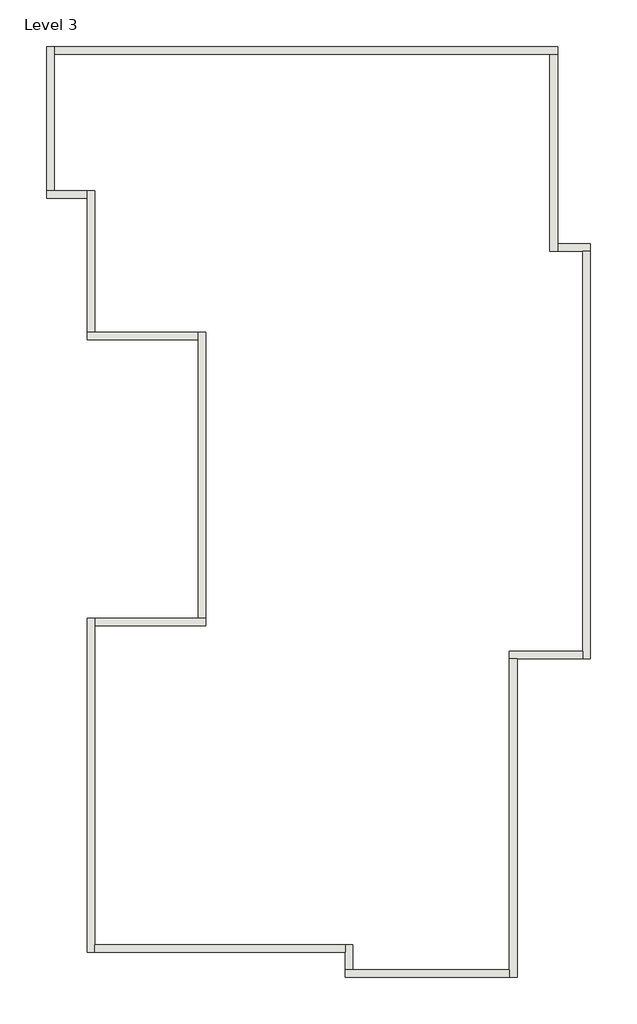
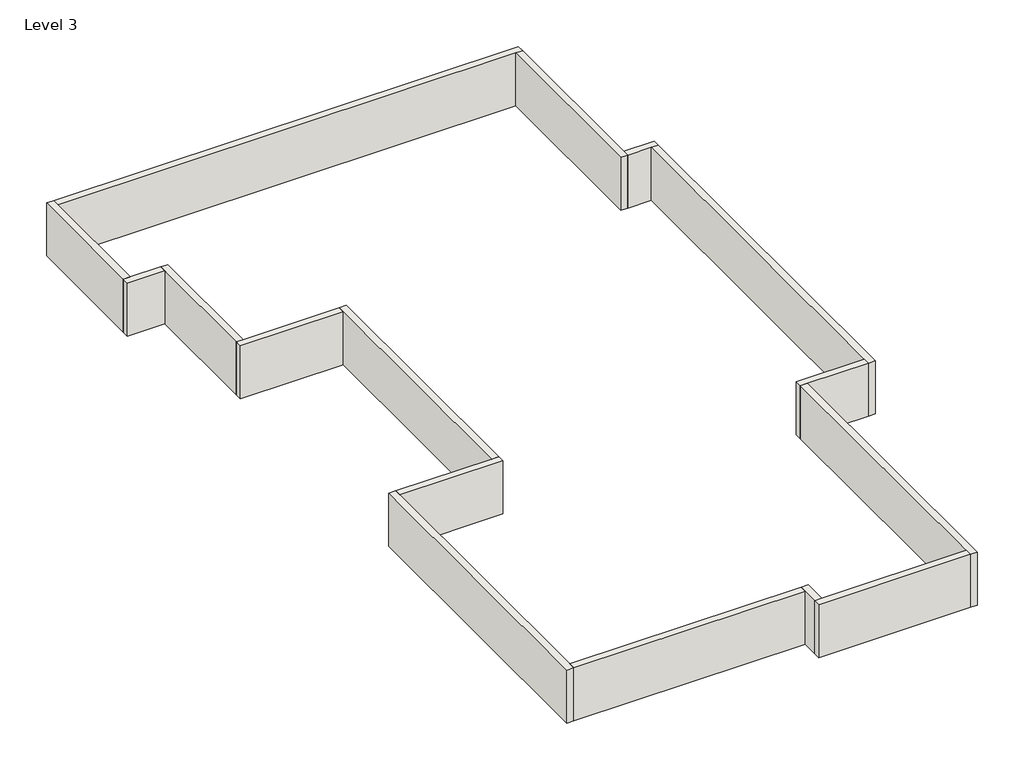
# One storey: 16 walls.
"""IFC4 building model written with IfcOpenShell, lengths in millimetres."""

from ifc_helpers import new_model, si_unit, frame, origin, place, context, project, spatial, polyline, outline, extrude, faceted_brep, element, save

model = new_model("IFC4")

# Units and contexts
model_context = context("Model", 3, world=origin())
ifc_project = project(units=[si_unit("LENGTHUNIT", "METRE", prefix="MILLI")], contexts=[model_context])

# Site, building, storey
site = spatial("IfcSite", under=ifc_project)
building = spatial("IfcBuilding", under=site)
storey = spatial("IfcBuildingStorey", under=building, Name="Level 3", Elevation=6400.8)

# Walls
placement = place(None, origin())
element("IfcWall", 1, ObjectType="Generic - 4.5\"", at=placement, inside=storey, context=model_context, shape_type="Brep", body=[
    faceted_brep([(-6988.9378503, -5768.8887643, 6400.8), (-6988.9378503, -5654.5887643, 6400.8), (-6988.9378503, -853.9864583, 6400.8), (-6988.9378503, -739.6864583, 6400.8), (-6988.9378503, -739.6864583, 7315.2), (-6988.9378503, -853.9864583, 7315.2), (-6988.9378503, -5654.5887643, 7315.2), (-6988.9378503, -5768.8887643, 7315.2), (-7103.2378503, -5768.8864583, 6400.8), (-7103.2378503, -5768.8864583, 7315.2), (-7103.2378503, -739.6864583, 7315.2), (-7103.2378503, -739.6864583, 6400.8)], [[[0, 1, 2, 3, 4, 5, 6, 7]], [[8, 9, 10, 11]], [[3, 2, 1, 0, 8, 11]], [[7, 6, 5, 4, 10, 9]], [[4, 3, 11, 10]], [[0, 7, 9, 8]]]),
])
element("IfcWall", 2, ObjectType="Generic - 4.5\"", at=placement, inside=storey, context=model_context, shape_type="Brep", body=[
    faceted_brep([(-6988.9378503, -853.9864583, 6400.8), (-5312.0457903, -853.9864583, 6400.8), (-5312.0457903, -853.9864583, 7315.2), (-6988.9378503, -853.9864583, 7315.2), (-6988.9378503, -739.6864583, 6400.8), (-6988.9378503, -739.6864583, 7315.2), (-5426.3457903, -739.6864583, 7315.2), (-5312.0457903, -739.6864583, 7315.2), (-5312.0457903, -739.6864583, 6400.8), (-5426.3457903, -739.6864583, 6400.8)], [[[0, 1, 2, 3]], [[4, 5, 6, 7, 8, 9]], [[1, 0, 4, 9, 8]], [[3, 2, 7, 6, 5]], [[0, 3, 5, 4]], [[2, 1, 8, 7]]]),
])
element("IfcWall", 3, ObjectType="Generic - 4.5\"", at=placement, inside=storey, context=model_context, shape_type="Brep", body=[
    faceted_brep([(-5312.0457903, -739.6864583, 6400.8), (-5312.0457903, 3565.6135417, 6400.8), (-5312.0457903, 3565.6135417, 7315.2), (-5312.0457903, -739.6864583, 7315.2), (-5426.3457903, -739.6864583, 6400.8), (-5426.3457903, -739.6864583, 7315.2), (-5426.3457903, 3451.3135417, 7315.2), (-5426.3457903, 3565.6135417, 7315.2), (-5426.3457903, 3565.6135417, 6400.8), (-5426.3457903, 3451.3135417, 6400.8)], [[[0, 1, 2, 3]], [[4, 5, 6, 7, 8, 9]], [[1, 0, 4, 9, 8]], [[3, 2, 7, 6, 5]], [[0, 3, 5, 4]], [[2, 1, 8, 7]]]),
])
element("IfcWall", 4, ObjectType="Generic - 4.5\"", at=placement, inside=storey, context=model_context, shape_type="Brep", body=[
    faceted_brep([(-5426.3457903, 3565.6135417, 6400.8), (-6988.9378503, 3565.6135417, 6400.8), (-7103.2378503, 3565.6135417, 6400.8), (-7103.2378503, 3565.6135417, 7315.2), (-6988.9378503, 3565.6135417, 7315.2), (-5426.3457903, 3565.6135417, 7315.2), (-5426.3457903, 3451.3135417, 6400.8), (-5426.3457903, 3451.3135417, 7315.2), (-7103.2378503, 3451.3135417, 7315.2), (-7103.2378503, 3451.3135417, 6400.8)], [[[0, 1, 2, 3, 4, 5]], [[6, 7, 8, 9]], [[2, 1, 0, 6, 9]], [[5, 4, 3, 8, 7]], [[0, 5, 7, 6]], [[3, 2, 9, 8]]]),
])
element("IfcWall", 5, ObjectType="Generic - 4.5\"", at=placement, inside=storey, context=model_context, shape_type="Brep", body=[
    faceted_brep([(-6988.9378503, 3565.6135417, 6400.8), (-6988.9378503, 5699.2135417, 6400.8), (-6988.9378503, 5699.2135417, 7315.2), (-6988.9378503, 3565.6135417, 7315.2), (-7103.2378503, 3565.6135417, 6400.8), (-7103.2378503, 3565.6135417, 7315.2), (-7103.2378503, 5584.9135417, 7315.2), (-7103.2378503, 5699.2135417, 7315.2), (-7103.2378503, 5699.2135417, 6400.8), (-7103.2378503, 5584.9135417, 6400.8)], [[[0, 1, 2, 3]], [[4, 5, 6, 7, 8, 9]], [[1, 0, 4, 9, 8]], [[3, 2, 7, 6, 5]], [[0, 3, 5, 4]], [[2, 1, 8, 7]]]),
])
element("IfcWall", 6, ObjectType="Generic - 4.5\"", at=placement, inside=storey, context=model_context, shape_type="Brep", body=[
    faceted_brep([(-7103.2378503, 5699.2135417, 6400.8), (-7598.5378503, 5699.2135417, 6400.8), (-7712.8378503, 5699.2135417, 6400.8), (-7712.8378503, 5699.2135417, 7315.2), (-7598.5378503, 5699.2135417, 7315.2), (-7103.2378503, 5699.2135417, 7315.2), (-7103.2378503, 5584.9135417, 6400.8), (-7103.2378503, 5584.9135417, 7315.2), (-7712.8378503, 5584.9135417, 7315.2), (-7712.8378503, 5584.9135417, 6400.8)], [[[0, 1, 2, 3, 4, 5]], [[6, 7, 8, 9]], [[2, 1, 0, 6, 9]], [[5, 4, 3, 8, 7]], [[0, 5, 7, 6]], [[3, 2, 9, 8]]]),
])
element("IfcWall", 7, ObjectType="Generic - 4.5\"", at=placement, inside=storey, context=model_context, shape_type="Brep", body=[
    faceted_brep([(-7598.5378503, 5699.2135417, 6400.8), (-7598.5378503, 7756.6135417, 6400.8), (-7598.5378503, 7870.9135417, 6400.8), (-7598.5378503, 7870.9135417, 7315.2), (-7598.5378503, 7756.6135417, 7315.2), (-7598.5378503, 5699.2135417, 7315.2), (-7712.8378503, 5699.2135417, 6400.8), (-7712.8378503, 5699.2135417, 7315.2), (-7712.8378503, 7870.9135417, 7315.2), (-7712.8378503, 7870.9135417, 6400.8)], [[[0, 1, 2, 3, 4, 5]], [[6, 7, 8, 9]], [[2, 1, 0, 6, 9]], [[5, 4, 3, 8, 7]], [[0, 5, 7, 6]], [[3, 2, 9, 8]]]),
])
element("IfcWall", 8, ObjectType="Generic - 4.5\"", at=placement, inside=storey, context=model_context, shape_type="Brep", body=[
    faceted_brep([(-7598.5378503, 7756.6135417, 6400.8), (-130.9378503, 7756.6135417, 6400.8), (-16.6378503, 7756.6135417, 6400.8), (-16.6378503, 7756.6135417, 7315.2), (-130.9378503, 7756.6135417, 7315.2), (-7598.5378503, 7756.6135417, 7315.2), (-7598.5378503, 7870.9135417, 6400.8), (-7598.5378503, 7870.9135417, 7315.2), (-16.6378503, 7870.9135417, 7315.2), (-16.6378503, 7870.9135417, 6400.8)], [[[0, 1, 2, 3, 4, 5]], [[6, 7, 8, 9]], [[2, 1, 0, 6, 9]], [[5, 4, 3, 8, 7]], [[0, 5, 7, 6]], [[3, 2, 9, 8]]]),
])
element("IfcWall", 9, ObjectType="Generic - 4.5\"", at=placement, inside=storey, context=model_context, shape_type="Brep", body=[
    faceted_brep([(-130.9378503, 7756.6135417, 6400.8), (-130.9378503, 4784.8135417, 6400.8), (-130.9378503, 4784.8135417, 7315.2), (-130.9378503, 7756.6135417, 7315.2), (-16.6378503, 7756.6135417, 6400.8), (-16.6378503, 7756.6135417, 7315.2), (-16.6378503, 4899.1135417, 7315.2), (-16.6378503, 4784.8135417, 7315.2), (-16.6378503, 4784.8135417, 6400.8), (-16.6378503, 4899.1135417, 6400.8)], [[[0, 1, 2, 3]], [[4, 5, 6, 7, 8, 9]], [[1, 0, 4, 9, 8]], [[3, 2, 7, 6, 5]], [[0, 3, 5, 4]], [[2, 1, 8, 7]]]),
])
element("IfcWall", 10, ObjectType="Generic - 4.5\"", at=placement, inside=storey, context=model_context, shape_type="Brep", body=[
    faceted_brep([(-16.6378503, 4784.8135417, 6400.8), (364.3621497, 4784.8135417, 6400.8), (478.6621497, 4784.8135417, 6400.8), (478.6621497, 4784.8135417, 7315.2), (364.3621497, 4784.8135417, 7315.2), (-16.6378503, 4784.8135417, 7315.2), (-16.6378503, 4899.1135417, 6400.8), (-16.6378503, 4899.1135417, 7315.2), (478.6621497, 4899.1135417, 7315.2), (478.6621497, 4899.1135417, 6400.8)], [[[0, 1, 2, 3, 4, 5]], [[6, 7, 8, 9]], [[2, 1, 0, 6, 9]], [[5, 4, 3, 8, 7]], [[0, 5, 7, 6]], [[3, 2, 9, 8]]]),
])
element("IfcWall", 11, ObjectType="Generic - 4.5\"", at=placement, inside=storey, context=model_context, shape_type="Brep", body=[
    faceted_brep([(364.3621497, 4784.8135417, 6400.8), (364.3621497, -1234.9864583, 6400.8), (364.3621497, -1349.2864583, 6400.8), (364.3621497, -1349.2864583, 7315.2), (364.3621497, -1234.9864583, 7315.2), (364.3621497, 4784.8135417, 7315.2), (478.6621497, 4784.8135417, 6400.8), (478.6621497, 4784.8135417, 7315.2), (478.6621497, -1349.2864583, 7315.2), (478.6621497, -1349.2864583, 6400.8)], [[[0, 1, 2, 3, 4, 5]], [[6, 7, 8, 9]], [[2, 1, 0, 6, 9]], [[5, 4, 3, 8, 7]], [[0, 5, 7, 6]], [[3, 2, 9, 8]]]),
])
element("IfcWall", 12, ObjectType="Generic - 4.5\"", at=placement, inside=storey, context=model_context, shape_type="Brep", body=[
    faceted_brep([(364.3621497, -1234.9864583, 6400.8), (-740.5378503, -1234.9864583, 6400.8), (-740.5378503, -1234.9864583, 7315.2), (364.3621497, -1234.9864583, 7315.2), (364.3621497, -1349.2864583, 6400.8), (364.3621497, -1349.2864583, 7315.2), (-626.2378503, -1349.2864583, 7315.2), (-740.5378503, -1349.2864583, 7315.2), (-740.5378503, -1349.2864583, 6400.8), (-626.2378503, -1349.2864583, 6400.8)], [[[0, 1, 2, 3]], [[4, 5, 6, 7, 8, 9]], [[1, 0, 4, 9, 8]], [[3, 2, 7, 6, 5]], [[0, 3, 5, 4]], [[2, 1, 8, 7]]]),
])
element("IfcWall", 13, ObjectType="Generic - 4.5\"", at=placement, inside=storey, context=model_context, shape_type="Brep", body=[
    faceted_brep([(-740.5378503, -1349.2864583, 6400.8), (-740.5378503, -6035.6648645, 6400.8), (-740.5378503, -6149.9648645, 6400.8), (-740.5378503, -6149.9648645, 7315.2), (-740.5378503, -6035.6648645, 7315.2), (-740.5378503, -1349.2864583, 7315.2), (-626.2378503, -1349.2864583, 6400.8), (-626.2378503, -1349.2864583, 7315.2), (-626.2378503, -6149.9648645, 7315.2), (-626.2378503, -6149.9648645, 6400.8)], [[[0, 1, 2, 3, 4, 5]], [[6, 7, 8, 9]], [[2, 1, 0, 6, 9]], [[5, 4, 3, 8, 7]], [[0, 5, 7, 6]], [[3, 2, 9, 8]]]),
])
element("IfcWall", 14, ObjectType="Generic - 4.5\"", at=placement, inside=storey, context=model_context, shape_type="Brep", body=[
    faceted_brep([(-740.5378503, -6035.6648645, 6400.8), (-3102.7378503, -6035.6648645, 6400.8), (-3217.0378503, -6035.6648645, 6400.8), (-3217.0378503, -6035.6648645, 7315.2), (-3102.7378503, -6035.6648645, 7315.2), (-740.5378503, -6035.6648645, 7315.2), (-740.5378503, -6149.9648645, 6400.8), (-740.5378503, -6149.9648645, 7315.2), (-3217.0378503, -6149.9648645, 7315.2), (-3217.0378503, -6149.9648645, 6400.8)], [[[0, 1, 2, 3, 4, 5]], [[6, 7, 8, 9]], [[2, 1, 0, 6, 9]], [[5, 4, 3, 8, 7]], [[0, 5, 7, 6]], [[3, 2, 9, 8]]]),
])
element("IfcWall", 15, ObjectType="Generic - 4.5\"", at=placement, inside=storey, context=model_context, shape_type="Brep", body=[
    faceted_brep([(-3102.7378503, -6035.6648645, 6400.8), (-3102.7378503, -5654.6671706, 6400.8), (-3102.7378503, -5654.6671706, 7315.2), (-3102.7378503, -6035.6648645, 7315.2), (-3217.0378503, -6035.6648645, 6400.8), (-3217.0378503, -6035.6648645, 7315.2), (-3217.0378503, -5768.9648645, 7315.2), (-3217.0378503, -5654.6648645, 7315.2), (-3217.0378503, -5654.6648645, 6400.8), (-3217.0378503, -5768.9648645, 6400.8)], [[[0, 1, 2, 3]], [[4, 5, 6, 7, 8, 9]], [[1, 0, 4, 9, 8]], [[3, 2, 7, 6, 5]], [[0, 3, 5, 4]], [[2, 1, 8, 7]]]),
])
element("IfcWall", 16, ObjectType="Generic - 4.5\"", at=placement, inside=storey, context=model_context, shape_type="SweptSolid", body=[
    extrude(outline(polyline([(-6988.9378503, -5654.5887643), (-3217.0378503, -5654.6648645), (-3217.0378503, -5768.9648645), (-6988.9378503, -5768.8887643), (-6988.9378503, -5654.5887643)])), frame((0.0, 0.0, 6400.8), z_axis=(0.0, 0.0, 1.0), x_axis=(1.0, 0.0, 0.0)), (0.0, 0.0, 1.0), 914.4),
])

save(model, "model.ifc")

# Revit data of these elements
# Type "Generic - 4.5\""
#   Assembly Code = "B2010"
#   Layers, outside or top first: 0' - 4 1/2" no material (function 1)
# Elements 1, 2, 3, 4, 5, 6, 7, 8, 9, 10, 11, 12, 13, 14, 15, 16 (IfcWall, "Generic - 4.5\"")
#   Top Offset = 0' - 0"
#   Base Offset = 0' - 0"
#   Unconnected Height = 3' - 0"
#   wall height = 3' - 0"
#   Phase Created = New Construction
#   Base Constraint = Level 3
#   Materials on its faces: "Default Wall", "Beige Colour"
# Materials
#   "Default Wall": colour RGB 128 128 128, transparency 0, Cost = 0
#   "Beige Colour": class "Generic", colour RGB 120 120 120, transparency 0, Cost = 0
